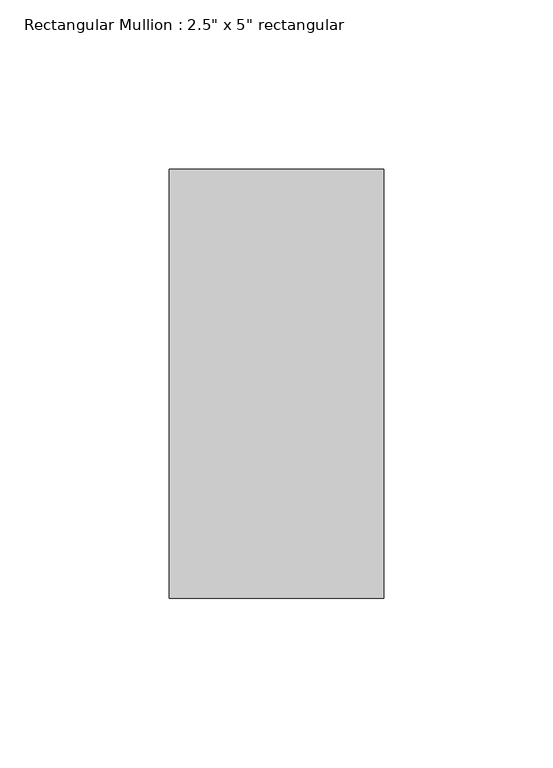
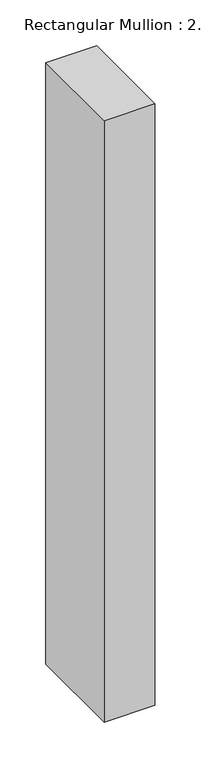
"""IFC4 building model written with IfcOpenShell, lengths in millimetres: member geometry."""

from ifc_helpers import new_model, si_unit, frame, origin, place, context, project, spatial, polyline, outline, extrude, source, transform, mapped, element, save


def member_ccd4d8c6(model_context):
    return source(origin(), model_context, "Body", "SweptSolid", [
        extrude(outline(polyline([(31.75, 63.5), (31.75, -63.5), (-31.75, -63.5), (-31.75, 63.5), (31.75, 63.5)])), frame((0.0, 0.0, -798.5443895), z_axis=(0.0, 0.0, 1.0), x_axis=(1.0, 0.0, 0.0)), (0.0, 0.0, 1.0), 798.5443895),
    ])


if __name__ == "__main__":
    model = new_model("IFC4")
    model_context = context("Model", 3, world=origin())
    ifc_project = project(units=[si_unit("LENGTHUNIT", "METRE", prefix="MILLI")], contexts=[model_context])
    site = spatial("IfcSite", under=ifc_project)
    building = spatial("IfcBuilding", under=site)
    placement = place(None, origin())
    member_shape = member_ccd4d8c6(model_context)
    element("IfcMember", 1, ObjectType="Rectangular Mullion : 2.5\" x 5\" rectangular", at=placement, inside=building, context=model_context, shape_type="MappedRepresentation", body=[
        mapped(member_shape, transform((0.0, 0.0, 0.0), x_axis=(1.0, 0.0, 0.0), y_axis=(0.0, 1.0, 0.0), z_axis=(0.0, 0.0, 1.0))),
    ])
    save(model, "model.ifc")

# Revit data of these elements
# Type "Rectangular Mullion : 2.5\" x 5\" rectangular"
#   built-in parameter 1007304 = 0.416667 (stored number, unit not read)
#   built-in parameter 1007301 = 0.104167 (stored number, unit not read)
#   built-in parameter 1007300 = 0.104167 (stored number, unit not read)
# Element 1 (IfcMember, "Rectangular Mullion : 2.5\" x 5\" rectangular")
#   Materials on its faces: "Aluminum"
# Materials
#   "Aluminum": class "Metal", colour RGB 247 247 247, transparency 0, Description = "Aluminum 6061", Cost = 0
